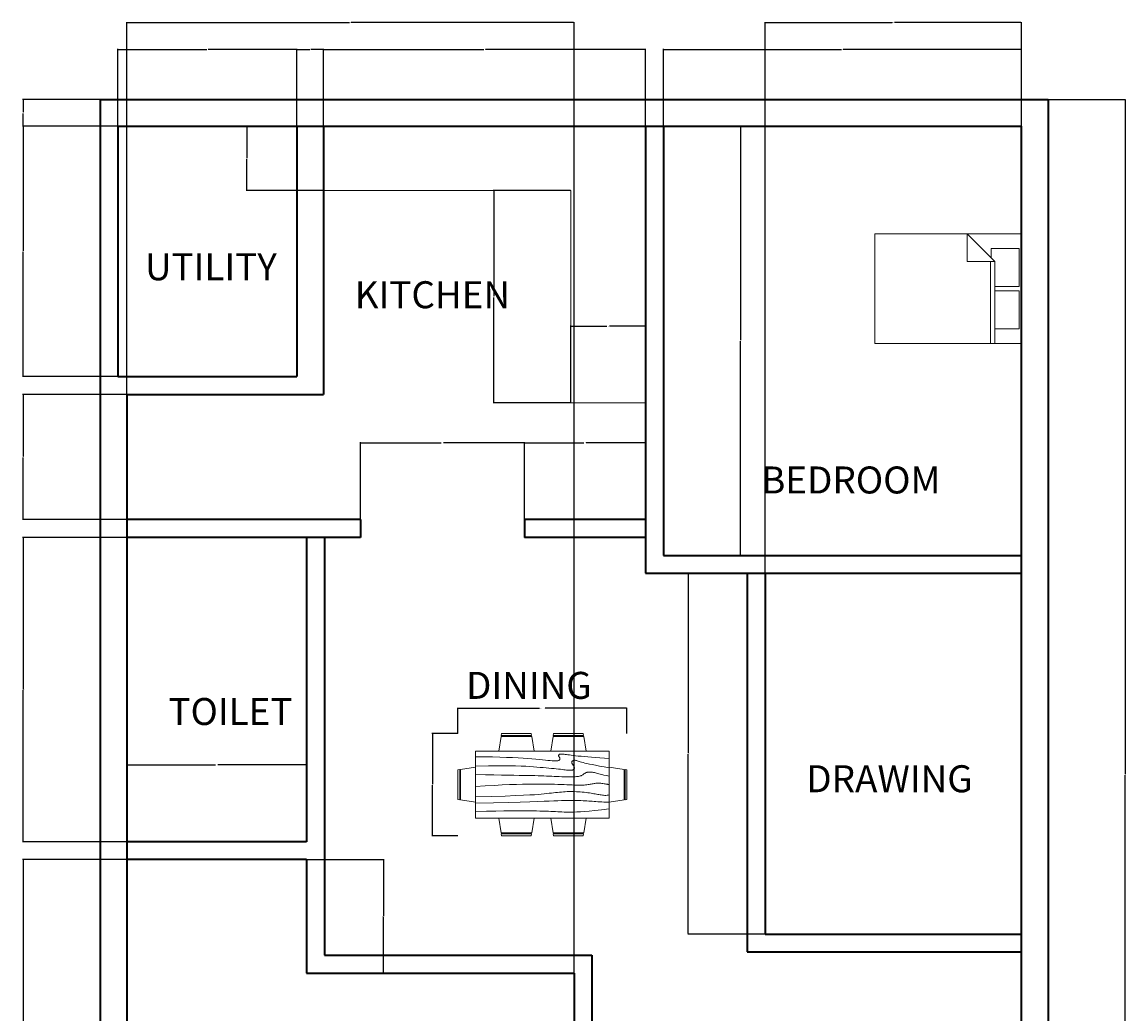
# Model space of a CAD drawing. Units: inches. Extents: x 3024 to 3952, y 1308 to 1863.
# Tile 29 of 29: x 3581 to 3952, y 1481 to 1814. Entities that reach past the tile are written whole.
import ezdxf

# ---------------------------------------------------------------- set-up
doc = ezdxf.new("R2010")
doc.units = ezdxf.units.IN
for name, color, linetype, lineweight in [('A-ANNO-DIMS', 2, 'Continuous', 18), ('A-AREA-IDEN', 7, 'Continuous', 18), ('A-FLOR-CASE', 8, 'Continuous', 18), ('A-FURN', 8, 'Continuous', 18), ('A-WALL', 7, 'Continuous', 35)]:
    doc.layers.add(name, color=color, linetype=linetype, lineweight=lineweight)
doc.styles.get("Standard").update_dxf_attribs({"font": 'arial.ttf'})
doc.dimstyles.get("Standard").update_dxf_attribs({"dimtxt": 0.18, "dimasz": 0.18, "dimexe": 0.18, "dimexo": 0.0625, "dimgap": 0.09, "dimtad": 0, "dimtih": 1, "dimtoh": 1, "dimdec": 4, "dimzin": 0, "dimdsep": 46, "dimtxsty": 'Standard', "dimcen": 0.09, "dimadec": 0, "dimazin": 0, "dimtfac": 1, "dimtdec": 4, "dimtofl": 0, "dimtmove": 0, "dimatfit": 3, "dimfxl": 1, "dimtolj": 1, "dimtzin": 0, "dimarcsym": 0})

# ---------------------------------------------------------------- blocks, each defined once
blk = doc.blocks.new('Bed - Queen')
for p, q in [((0, -80.00003), (0, 0)), ((0, 0), (59.99999, 0)), ((59.99999, 0), (59.99999, -80.00003)), ((7.99999, -1.2), (28.79998, -1.2)), ((7.99999, -14.4), (7.99999, -1.2)), ((28.79998, -1.2), (28.79998, -14.4)), ((31.19999, -1.2), (51.99999, -1.2)), ((31.19999, -14.4), (31.19999, -1.2)), ((51.99999, -1.2), (51.99999, -16.4)), ((0, -14.4), (44.8, -14.4)), ((44.8, -16.8), (0, -16.8)), ((59.99999, -29.6), (44.8, -14.4)), ((44.8, -14.4), (44.8, -29.6)), ((51.99999, -16.4), (46.79936, -16.4)), ((44.8, -29.6), (59.99999, -29.6)), ((59.99999, -80.00003), (0, -80.00003))]:
    blk.add_line(p, q)
blk = doc.blocks.new('Dining Set - 36 x 72 in.')
for p, q in [((-22.2343, 26.00059), (-23.4847, 17.99762)), ((-22.2304, 26), (-5.7608, 26)), ((-22, 27.5), (-22.1562, 26.50042)), ((-5.8416, 26.5), (-22.1534, 26.5)), ((-22, 27.5), (-6, 27.5)), ((-5.8437, 26.49966), (-6, 27.5)), ((-4.5152, 17.99762), (-5.7655, 25.99926)), ((5.7657, 26.00059), (4.5153, 17.99762)), ((5.7696, 26), (22.2392, 26)), ((6, 27.5), (5.8438, 26.50042)), ((22.1584, 26.5), (5.8466, 26.5)), ((6, 27.5), (22, 27.5)), ((22.1563, 26.49966), (22, 27.5)), ((23.4848, 17.99762), (22.2345, 25.99926)), ((36, 18), (-36, 18)), ((-36, 18), (-36, -18)), ((36, -18), (36, 18)), ((-45.5, 8), (-44.5004, 8.15617)), ((-45.5, 8), (-45.5, -8)), ((-44.5, -8.15843), (-44.5, 8.15338)), ((-44.0006, 8.23428), (-35.9976, 9.48474)), ((-44, 8.23041), (-44, -8.23915)), ((44.0006, 8.23428), (35.9976, 9.48474)), ((44, 8.23041), (44, -8.23915)), ((44.5, -8.15843), (44.5, 8.15338)), ((45.5, 8), (44.5005, 8.15617)), ((45.5, 8), (45.5, -8)), ((-44.4997, -8.15631), (-45.5, -8)), ((-35.9976, -9.48476), (-43.9993, -8.2345)), ((35.9976, -9.48476), (43.9993, -8.2345)), ((44.4997, -8.15631), (45.5, -8)), ((-36, -18), (36, -18)), ((-22.2343, -26.0006), (-23.4847, -17.99762)), ((-4.5152, -17.99762), (-5.7655, -25.99928)), ((5.7657, -26.0006), (4.5153, -17.99762)), ((23.4848, -17.99762), (22.2345, -25.99928)), ((-22.2304, -26), (-5.7608, -26)), ((-22, -27.5), (-22.1562, -26.50044)), ((-5.8416, -26.5), (-22.1534, -26.5)), ((-22, -27.5), (-6, -27.5)), ((-5.8437, -26.49967), (-6, -27.5)), ((5.7696, -26), (22.2392, -26)), ((6, -27.5), (5.8438, -26.50044)), ((22.1584, -26.5), (5.8466, -26.5)), ((6, -27.5), (22, -27.5)), ((22.1563, -26.49967), (22, -27.5))]:
    blk.add_line(p, q)
for points in [[(-36, 15), (-31.1772, 14.97754), (-26.8079, 14.91406), (-22.8538, 14.81543), (-19.276, 14.6875), (-16.0362, 14.53613), (-13.0957, 14.36718), (-10.4159, 14.18652), (-7.9583, 14), (-5.6904, 13.81315), (-3.6035, 13.63021), (-1.6954, 13.45508), (0.0365, 13.29166), (1.5945, 13.14388), (2.9811, 13.01562), (4.1988, 12.9108), (5.25, 12.83333), (6.1393, 12.78613), (6.8802, 12.76823), (7.4883, 12.77767), (7.9792, 12.8125), (8.3685, 12.87077), (8.6719, 12.95052), (8.9049, 13.0498), (9.0833, 13.16666), (9.2205, 13.29899), (9.3216, 13.44401), (9.3895, 13.59879), (9.4271, 13.76041), (9.4373, 13.92594), (9.4232, 14.09245), (9.3875, 14.257), (9.3333, 14.41666), (9.2638, 14.56917), (9.1836, 14.71484), (9.0975, 14.85465), (9.0104, 14.98958), (8.9272, 15.1206), (8.8529, 15.2487), (8.7922, 15.37483), (8.75, 15.5), (8.7305, 15.62467), (8.7344, 15.74739), (8.7617, 15.86621), (8.8125, 15.97916), (8.8867, 16.08431), (8.9844, 16.17968), (9.1055, 16.26334), (9.25, 16.33333), (9.4189, 16.38802), (9.6172, 16.42708), (9.8506, 16.45052), (10.125, 16.45833), (10.4463, 16.45052), (10.8203, 16.42708), (11.2529, 16.38802), (11.75, 16.33333), (12.3184, 16.26318), (12.9694, 16.17838), (13.7151, 16.07991), (14.5677, 15.96875), (15.5395, 15.84586), (16.6426, 15.71224), (17.8893, 15.56884), (19.2917, 15.41666), (20.859, 15.25667), (22.5879, 15.08984), (24.4721, 14.91715), (26.5052, 14.73958), (28.6809, 14.5581), (30.9929, 14.3737), (33.4347, 14.18733), (36, 14)], [(-36, 10), (-28.9766, 10.14274), (-23.1725, 10.20442), (-18.4241, 10.19775), (-14.5677, 10.13541), (-11.4399, 10.03011), (-8.877, 9.89453), (-6.7154, 9.74137), (-4.7917, 9.58333), (-2.9698, 9.43082), (-1.2246, 9.28515), (0.4415, 9.14534), (2.026, 9.01041), (3.5266, 8.87939), (4.9408, 8.7513), (6.266, 8.62516), (7.5, 8.5), (8.6411, 8.37549), (9.6914, 8.2539), (10.6538, 8.13818), (11.5312, 8.03125), (12.3267, 7.93603), (13.043, 7.85547), (13.6831, 7.79248), (14.25, 7.75), (14.7471, 7.7303), (15.1797, 7.73307), (15.5537, 7.75732), (15.875, 7.80208), (16.1494, 7.86637), (16.3828, 7.94922), (16.5811, 8.04964), (16.75, 8.16666), (16.8944, 8.29915), (17.0143, 8.44531), (17.1089, 8.60319), (17.1771, 8.77083), (17.218, 8.94629), (17.2305, 9.1276), (17.2137, 9.31282), (17.1667, 9.5), (17.0895, 9.6875), (16.987, 9.875), (16.8649, 10.0625), (16.7292, 10.25), (16.5856, 10.4375), (16.4401, 10.625), (16.2985, 10.8125), (16.1667, 11), (16.05, 11.18733), (15.9518, 11.3737), (15.8752, 11.5581), (15.8229, 11.73958), (15.798, 11.91715), (15.8034, 12.08984), (15.842, 12.25667), (15.9167, 12.41666), (16.0295, 12.56836), (16.1784, 12.70833), (16.3605, 12.83268), (16.5729, 12.9375), (16.8127, 13.01888), (17.0768, 13.07291), (17.3625, 13.0957), (17.6667, 13.08333), (17.9894, 13.03312), (18.3418, 12.94726), (18.7382, 12.82918), (19.1927, 12.68229), (19.7195, 12.51001), (20.3327, 12.31575), (21.0465, 12.10294), (21.875, 11.875), (22.8357, 11.63354), (23.959, 11.37304), (25.2786, 11.08618), (26.8282, 10.76562), (28.6414, 10.40405), (30.752, 9.99414), (33.1936, 9.52856), (36, 9)], [(-36, 5.5), (-30.7157, 5.3348), (-26.069, 5.20963), (-21.9946, 5.11767), (-18.4271, 5.05208), (-15.3009, 5.00602), (-12.5508, 4.97265), (-10.1112, 4.94515), (-7.9167, 4.91666), (-5.909, 4.88167), (-4.0586, 4.83984), (-2.3429, 4.79215), (-0.7396, 4.73958), (0.7739, 4.6831), (2.22, 4.6237), (3.6213, 4.56233), (5, 4.5), (6.373, 4.43782), (7.7344, 4.3776), (9.0723, 4.32129), (10.375, 4.27083), (11.6309, 4.22819), (12.8281, 4.19531), (13.9551, 4.17415), (15, 4.16666), (15.954, 4.17448), (16.819, 4.19791), (17.6001, 4.23698), (18.3021, 4.29166), (18.9299, 4.36198), (19.4883, 4.44791), (19.9823, 4.54948), (20.4167, 4.66666), (20.7969, 4.79899), (21.1302, 4.94401), (21.4245, 5.09879), (21.6875, 5.26041), (21.9271, 5.42594), (22.1511, 5.59245), (22.3672, 5.757), (22.5834, 5.91666), (22.8065, 6.06868), (23.0404, 6.21093), (23.2879, 6.34147), (23.5521, 6.45833), (23.8358, 6.55957), (24.142, 6.64323), (24.4735, 6.70735), (24.8334, 6.75), (25.2235, 6.76969), (25.642, 6.76692), (26.0858, 6.74267), (26.5521, 6.69791), (27.0379, 6.63362), (27.5404, 6.55078), (28.0565, 6.45036), (28.5834, 6.33333), (29.1242, 6.19987), (29.7071, 6.04687), (30.3661, 5.87044), (31.1354, 5.66666), (32.0493, 5.43164), (33.142, 5.16146), (34.4475, 4.85221), (36, 4.5)], [(-36, -1), (-30.7915, -0.6591), (-26.0195, -0.38216), (-21.6519, -0.16284), (-17.6563, 0.00521), (-14.0005, 0.12833), (-10.6523, 0.21289), (-7.5796, 0.26522), (-4.75, 0.29166), (-2.134, 0.29793), (0.2878, 0.28711), (2.5317, 0.26163), (4.6146, 0.22396), (6.5529, 0.17651), (8.3633, 0.12174), (10.0623, 0.06209), (11.6667, 0), (13.1899, -0.06201), (14.6341, -0.1211), (15.9982, -0.17432), (17.2813, -0.21875), (18.4823, -0.25147), (19.6003, -0.26953), (20.6343, -0.27002), (21.5834, -0.25), (22.4481, -0.20768), (23.2357, -0.14584), (23.9549, -0.06836), (24.6146, 0.02083), (25.2235, 0.11784), (25.7904, 0.21875), (26.3241, 0.31966), (26.8334, 0.41666), (27.3265, 0.50618), (27.8099, 0.58593), (28.2894, 0.65397), (28.7709, 0.70833), (29.2601, 0.74707), (29.763, 0.76823), (30.2855, 0.76985), (30.8334, 0.75), (31.4088, 0.70784), (31.9994, 0.64713), (32.589, 0.57275), (33.1615, 0.48958), (33.7008, 0.4025), (34.1908, 0.3164), (34.6153, 0.23616), (34.9584, 0.16666), (35.2099, 0.11165), (35.3848, 0.07031), (35.504, 0.04069), (35.5886, 0.02083), (35.6594, 0.00879), (35.7377, 0.0026), (35.8442, 0.00032), (36, 0)], [(-36, -6.5), (-27.1843, -6.31267), (-20.084, -6.1263), (-14.469, -5.9419), (-10.1094, -5.76042), (-6.7752, -5.58285), (-4.2363, -5.41016), (-2.2629, -5.24333), (-0.625, -5.08334), (0.8708, -4.93099), (2.2715, -4.78646), (3.5872, -4.64974), (4.8281, -4.52084), (6.0046, -4.39974), (7.127, -4.28646), (8.2053, -4.18099), (9.25, -4.08334), (10.2705, -3.99382), (11.2734, -3.91407), (12.2647, -3.84603), (13.25, -3.79167), (14.2354, -3.75293), (15.2266, -3.73177), (16.2295, -3.73015), (17.25, -3.75), (18.2912, -3.79248), (19.3451, -3.85547), (20.4009, -3.93604), (21.4479, -4.03125), (22.4754, -4.13819), (23.4727, -4.25391), (24.4289, -4.37549), (25.3334, -4.5), (26.1785, -4.62492), (26.9694, -4.74935), (27.7145, -4.87281), (28.4219, -4.99479), (29.1, -5.11483), (29.7572, -5.23242), (30.4016, -5.34709), (31.0417, -5.45834), (31.6837, -5.56437), (32.3262, -5.65821), (32.9658, -5.73153), (33.599, -5.77604), (34.2224, -5.78345), (34.8327, -5.74545), (35.4264, -5.65373), (36, -5.5)], [(-36, -10), (-26.4022, -9.81299), (-18.4675, -9.62891), (-11.9839, -9.45069), (-6.7396, -9.28125), (-2.5226, -9.12354), (0.8789, -8.98047), (3.6769, -8.85498), (6.0833, -8.75), (8.2767, -8.66765), (10.3021, -8.60677), (12.1712, -8.56543), (13.8958, -8.54167), (15.4876, -8.53353), (16.9583, -8.53907), (18.3197, -8.55632), (19.5834, -8.58334), (20.7616, -8.61841), (21.8685, -8.66081), (22.9188, -8.71004), (23.9271, -8.76563), (24.9081, -8.82707), (25.8763, -8.89388), (26.8465, -8.96558), (27.8334, -9.04167), (28.8474, -9.12118), (29.8828, -9.20117), (30.93, -9.27824), (31.9792, -9.34896), (33.0205, -9.40991), (34.0443, -9.45768), (35.0407, -9.48885), (36, -9.5)], [(-36, -14.5), (-30.0881, -14.33513), (-25.0332, -14.21224), (-20.7312, -14.12647), (-17.0781, -14.07292), (-13.97, -14.04671), (-11.3027, -14.04297), (-8.9724, -14.05681), (-6.875, -14.08334), (-4.9224, -14.11833), (-3.0905, -14.16016), (-1.3709, -14.20785), (0.2448, -14.26042), (1.7647, -14.3169), (3.1973, -14.3763), (4.5507, -14.43767), (5.8333, -14.5), (7.0554, -14.5621), (8.235, -14.62175), (9.3922, -14.67652), (10.5469, -14.72396), (11.7192, -14.76164), (12.929, -14.78711), (14.1965, -14.79794), (15.5417, -14.79167), (16.9933, -14.76424), (18.6152, -14.70508), (20.4804, -14.60197), (22.6615, -14.44271), (25.2312, -14.21509), (28.2624, -13.9069), (31.8277, -13.50594), (36, -13)]]:
    blk.add_lwpolyline(points)
blk = doc.blocks.new('*D22')
at = {"layer": 'A-ANNO-DIMS', "color": 0, "lineweight": -2, "transparency": 16777216}
for p, q in [((3727.65, 1574.87), (3727.65, 1583.49)), ((3727.83, 1583.31), (3755.04, 1583.31)), ((3784.17, 1583.31), (3756.97, 1583.31)), ((3784.35, 1574.87), (3784.35, 1583.49))]:
    blk.add_line(p, q, dxfattribs=at)
at = {"layer": 'A-ANNO-DIMS', "color": 0, "transparency": 16777216}
for points in [[(3727.83, 1583.34), (3727.83, 1583.28), (3727.65, 1583.31)], [(3784.17, 1583.34), (3784.17, 1583.28), (3784.35, 1583.31)]]:
    blk.add_solid(points, dxfattribs=at)
at = {"layer": 'Defpoints', "color": 0, "transparency": 16777216}
for p in [(3784.35, 1583.31), (3727.65, 1574.81), (3784.35, 1574.81)]:
    blk.add_point(p, dxfattribs=at)
at = {"layer": 'A-ANNO-DIMS', "color": 0, "transparency": 16777216, "insert": (3756, 1583.31), "char_height": 0.18, "attachment_point": 5}
blk.add_mtext('\\A1;DINING SET 57', dxfattribs=at)
blk = doc.blocks.new('*D23')
at = {"layer": 'A-ANNO-DIMS', "color": 0, "lineweight": -2, "transparency": 16777216}
for p, q in [((3727.59, 1574.81), (3718.97, 1574.81)), ((3719.15, 1574.63), (3719.15, 1557.85)), ((3719.15, 1540.72), (3719.15, 1557.49)), ((3727.59, 1540.54), (3718.97, 1540.54))]:
    blk.add_line(p, q, dxfattribs=at)
at = {"layer": 'A-ANNO-DIMS', "color": 0, "transparency": 16777216}
for points in [[(3719.12, 1574.63), (3719.18, 1574.63), (3719.15, 1574.81)], [(3719.12, 1540.72), (3719.18, 1540.72), (3719.15, 1540.54)]]:
    blk.add_solid(points, dxfattribs=at)
at = {"layer": 'Defpoints', "color": 0, "transparency": 16777216}
for p in [(3719.15, 1574.81), (3727.65, 1574.81), (3727.65, 1540.54)]:
    blk.add_point(p, dxfattribs=at)
at = {"layer": 'A-ANNO-DIMS', "color": 0, "transparency": 16777216, "insert": (3719.15, 1557.67), "char_height": 0.18, "attachment_point": 5}
blk.add_mtext('\\A1;34', dxfattribs=at)
blk = doc.blocks.new('*D82')
at = {"layer": 'A-ANNO-DIMS', "color": 0, "lineweight": -2, "transparency": 16777216}
for p, q in [((3925.7, 1787.61), (3951.59, 1787.61)), ((3951.41, 1787.43), (3951.41, 1561.21)), ((3951.41, 1334.62), (3951.41, 1560.84)), ((3925.7, 1334.44), (3951.59, 1334.44))]:
    blk.add_line(p, q, dxfattribs=at)
at = {"layer": 'A-ANNO-DIMS', "color": 0, "transparency": 16777216}
for points in [[(3951.38, 1787.43), (3951.44, 1787.43), (3951.41, 1787.61)], [(3951.38, 1334.62), (3951.44, 1334.62), (3951.41, 1334.44)]]:
    blk.add_solid(points, dxfattribs=at)
at = {"layer": 'Defpoints', "color": 0, "transparency": 16777216}
for p in [(3925.64, 1787.61), (3951.41, 1787.61), (3925.64, 1334.44)]:
    blk.add_point(p, dxfattribs=at)
at = {"layer": 'A-ANNO-DIMS', "color": 0, "transparency": 16777216, "insert": (3951.41, 1561.02), "char_height": 0.18, "attachment_point": 5}
blk.add_mtext('\\A1;453.2', dxfattribs=at)
blk = doc.blocks.new('*D83')
at = {"layer": 'A-ANNO-DIMS', "color": 0, "lineweight": -2, "transparency": 16777216}
for p, q in [((3613.64, 1778.67), (3613.64, 1804.56)), ((3613.82, 1804.38), (3643.42, 1804.38)), ((3673.46, 1804.38), (3643.86, 1804.38)), ((3673.64, 1778.67), (3673.64, 1804.56))]:
    blk.add_line(p, q, dxfattribs=at)
at = {"layer": 'A-ANNO-DIMS', "color": 0, "transparency": 16777216}
for points in [[(3613.82, 1804.41), (3613.82, 1804.35), (3613.64, 1804.38)], [(3673.46, 1804.41), (3673.46, 1804.35), (3673.64, 1804.38)]]:
    blk.add_solid(points, dxfattribs=at)
at = {"layer": 'Defpoints', "color": 0, "transparency": 16777216}
for p in [(3673.64, 1804.38), (3613.64, 1778.61), (3673.64, 1778.61)]:
    blk.add_point(p, dxfattribs=at)
at = {"layer": 'A-ANNO-DIMS', "color": 0, "transparency": 16777216, "insert": (3643.64, 1804.38), "char_height": 0.18, "attachment_point": 5}
blk.add_mtext('\\A1;60', dxfattribs=at)
blk = doc.blocks.new('*D84')
at = {"layer": 'A-ANNO-DIMS', "color": 0, "lineweight": -2, "transparency": 16777216}
for p, q in [((3682.64, 1778.67), (3682.64, 1804.56)), ((3682.82, 1804.38), (3736.36, 1804.38)), ((3790.46, 1804.38), (3736.92, 1804.38)), ((3790.64, 1778.67), (3790.64, 1804.56))]:
    blk.add_line(p, q, dxfattribs=at)
at = {"layer": 'A-ANNO-DIMS', "color": 0, "transparency": 16777216}
for points in [[(3682.82, 1804.41), (3682.82, 1804.35), (3682.64, 1804.38)], [(3790.46, 1804.41), (3790.46, 1804.35), (3790.64, 1804.38)]]:
    blk.add_solid(points, dxfattribs=at)
at = {"layer": 'Defpoints', "color": 0, "transparency": 16777216}
for p in [(3790.64, 1804.38), (3682.64, 1778.61), (3790.64, 1778.61)]:
    blk.add_point(p, dxfattribs=at)
at = {"layer": 'A-ANNO-DIMS', "color": 0, "transparency": 16777216, "insert": (3736.64, 1804.38), "char_height": 0.18, "attachment_point": 5}
blk.add_mtext('\\A1;108', dxfattribs=at)
blk = doc.blocks.new('*D85')
at = {"layer": 'A-ANNO-DIMS', "color": 0, "lineweight": -2, "transparency": 16777216}
for p, q in [((3796.64, 1778.67), (3796.64, 1804.56)), ((3796.82, 1804.38), (3856.36, 1804.38)), ((3916.46, 1804.38), (3856.92, 1804.38)), ((3916.64, 1778.67), (3916.64, 1804.56))]:
    blk.add_line(p, q, dxfattribs=at)
at = {"layer": 'A-ANNO-DIMS', "color": 0, "transparency": 16777216}
for points in [[(3796.82, 1804.41), (3796.82, 1804.35), (3796.64, 1804.38)], [(3916.46, 1804.41), (3916.46, 1804.35), (3916.64, 1804.38)]]:
    blk.add_solid(points, dxfattribs=at)
at = {"layer": 'Defpoints', "color": 0, "transparency": 16777216}
for p in [(3916.64, 1804.38), (3796.64, 1778.61), (3916.64, 1778.61)]:
    blk.add_point(p, dxfattribs=at)
at = {"layer": 'A-ANNO-DIMS', "color": 0, "transparency": 16777216, "insert": (3856.64, 1804.38), "char_height": 0.18, "attachment_point": 5}
blk.add_mtext('\\A1;120', dxfattribs=at)
blk = doc.blocks.new('*D86')
at = {"layer": 'A-ANNO-DIMS', "color": 0, "lineweight": -2, "transparency": 16777216}
for p, q in [((3613.58, 1778.61), (3581.68, 1778.61)), ((3581.86, 1778.43), (3581.86, 1736.79)), ((3581.86, 1694.79), (3581.86, 1736.42)), ((3613.58, 1694.61), (3581.68, 1694.61))]:
    blk.add_line(p, q, dxfattribs=at)
at = {"layer": 'A-ANNO-DIMS', "color": 0, "transparency": 16777216}
for points in [[(3581.83, 1778.43), (3581.89, 1778.43), (3581.86, 1778.61)], [(3581.83, 1694.79), (3581.89, 1694.79), (3581.86, 1694.61)]]:
    blk.add_solid(points, dxfattribs=at)
at = {"layer": 'Defpoints', "color": 0, "transparency": 16777216}
for p in [(3613.64, 1778.61), (3581.86, 1694.61), (3613.64, 1694.61)]:
    blk.add_point(p, dxfattribs=at)
at = {"layer": 'A-ANNO-DIMS', "color": 0, "transparency": 16777216, "insert": (3581.86, 1736.61), "char_height": 0.18, "attachment_point": 5}
blk.add_mtext('\\A1;84', dxfattribs=at)
blk = doc.blocks.new('*D87')
at = {"layer": 'A-ANNO-DIMS', "color": 0, "lineweight": -2, "transparency": 16777216}
for p, q in [((3616.58, 1688.61), (3581.68, 1688.61)), ((3581.86, 1688.43), (3581.86, 1667.79)), ((3581.86, 1646.79), (3581.86, 1667.43)), ((3616.58, 1646.61), (3581.68, 1646.61))]:
    blk.add_line(p, q, dxfattribs=at)
at = {"layer": 'A-ANNO-DIMS', "color": 0, "transparency": 16777216}
for points in [[(3581.83, 1688.43), (3581.89, 1688.43), (3581.86, 1688.61)], [(3581.83, 1646.79), (3581.89, 1646.79), (3581.86, 1646.61)]]:
    blk.add_solid(points, dxfattribs=at)
at = {"layer": 'Defpoints', "color": 0, "transparency": 16777216}
for p in [(3616.64, 1688.61), (3581.86, 1646.61), (3616.64, 1646.61)]:
    blk.add_point(p, dxfattribs=at)
at = {"layer": 'A-ANNO-DIMS', "color": 0, "transparency": 16777216, "insert": (3581.86, 1667.61), "char_height": 0.18, "attachment_point": 5}
blk.add_mtext('\\A1;42', dxfattribs=at)
blk = doc.blocks.new('*D88')
at = {"layer": 'A-ANNO-DIMS', "color": 0, "lineweight": -2, "transparency": 16777216}
for p, q in [((3796.7, 1778.61), (3822.59, 1778.61)), ((3822.41, 1778.43), (3822.41, 1706.79)), ((3822.41, 1634.79), (3822.41, 1706.43)), ((3796.7, 1634.61), (3822.59, 1634.61))]:
    blk.add_line(p, q, dxfattribs=at)
at = {"layer": 'A-ANNO-DIMS', "color": 0, "transparency": 16777216}
for points in [[(3822.38, 1778.43), (3822.44, 1778.43), (3822.41, 1778.61)], [(3822.38, 1634.79), (3822.44, 1634.79), (3822.41, 1634.61)]]:
    blk.add_solid(points, dxfattribs=at)
at = {"layer": 'Defpoints', "color": 0, "transparency": 16777216}
for p in [(3796.64, 1778.61), (3796.64, 1634.61), (3822.41, 1634.61)]:
    blk.add_point(p, dxfattribs=at)
at = {"layer": 'A-ANNO-DIMS', "color": 0, "transparency": 16777216, "insert": (3822.41, 1706.61), "char_height": 0.18, "attachment_point": 5}
blk.add_mtext('\\A1;144', dxfattribs=at)
blk = doc.blocks.new('*D89')
at = {"layer": 'A-ANNO-DIMS', "color": 0, "lineweight": -2, "transparency": 16777216}
for p, q in [((3830.66, 1628.61), (3804.77, 1628.61)), ((3804.95, 1628.43), (3804.95, 1568.25)), ((3804.95, 1507.7), (3804.95, 1567.88)), ((3830.66, 1507.52), (3804.77, 1507.52))]:
    blk.add_line(p, q, dxfattribs=at)
at = {"layer": 'A-ANNO-DIMS', "color": 0, "transparency": 16777216}
for points in [[(3804.92, 1628.43), (3804.98, 1628.43), (3804.95, 1628.61)], [(3804.92, 1507.7), (3804.98, 1507.7), (3804.95, 1507.52)]]:
    blk.add_solid(points, dxfattribs=at)
at = {"layer": 'Defpoints', "color": 0, "transparency": 16777216}
for p in [(3804.95, 1628.61), (3830.72, 1628.61), (3830.72, 1507.52)]:
    blk.add_point(p, dxfattribs=at)
at = {"layer": 'A-ANNO-DIMS', "color": 0, "transparency": 16777216, "insert": (3804.95, 1568.06), "char_height": 0.18, "attachment_point": 5}
blk.add_mtext('\\A1;121.08', dxfattribs=at)
blk = doc.blocks.new('*D90')
at = {"layer": 'A-ANNO-DIMS', "color": 0, "lineweight": -2, "transparency": 16777216}
for p, q in [((3830.72, 1507.58), (3830.72, 1813.56)), ((3830.9, 1813.38), (3873.29, 1813.38)), ((3916.46, 1813.38), (3874.07, 1813.38)), ((3916.64, 1507.58), (3916.64, 1813.56))]:
    blk.add_line(p, q, dxfattribs=at)
at = {"layer": 'A-ANNO-DIMS', "color": 0, "transparency": 16777216}
for points in [[(3830.9, 1813.41), (3830.9, 1813.35), (3830.72, 1813.38)], [(3916.46, 1813.41), (3916.46, 1813.35), (3916.64, 1813.38)]]:
    blk.add_solid(points, dxfattribs=at)
at = {"layer": 'Defpoints', "color": 0, "transparency": 16777216}
for p in [(3916.64, 1813.38), (3830.72, 1507.52), (3916.64, 1507.52)]:
    blk.add_point(p, dxfattribs=at)
at = {"layer": 'A-ANNO-DIMS', "color": 0, "transparency": 16777216, "insert": (3873.68, 1813.38), "char_height": 0.18, "attachment_point": 5}
blk.add_mtext('\\A1;85.92', dxfattribs=at)
blk = doc.blocks.new('*D91')
at = {"layer": 'A-ANNO-DIMS', "color": 0, "lineweight": -2, "transparency": 16777216}
for p, q in [((3616.64, 1538.58), (3616.64, 1564.48)), ((3616.82, 1564.3), (3646.39, 1564.3)), ((3676.74, 1564.3), (3647.17, 1564.3)), ((3676.92, 1538.58), (3676.92, 1564.48))]:
    blk.add_line(p, q, dxfattribs=at)
at = {"layer": 'A-ANNO-DIMS', "color": 0, "transparency": 16777216}
for points in [[(3616.82, 1564.33), (3616.82, 1564.27), (3616.64, 1564.3)], [(3676.74, 1564.33), (3676.74, 1564.27), (3676.92, 1564.3)]]:
    blk.add_solid(points, dxfattribs=at)
at = {"layer": 'Defpoints', "color": 0, "transparency": 16777216}
for p in [(3676.92, 1564.3), (3616.64, 1538.52), (3676.92, 1538.52)]:
    blk.add_point(p, dxfattribs=at)
at = {"layer": 'A-ANNO-DIMS', "color": 0, "transparency": 16777216, "insert": (3646.78, 1564.3), "char_height": 0.18, "attachment_point": 5}
blk.add_mtext('\\A1;60.28', dxfattribs=at)
blk = doc.blocks.new('*D92')
at = {"layer": 'A-ANNO-DIMS', "color": 0, "lineweight": -2, "transparency": 16777216}
for p, q in [((3616.58, 1640.61), (3581.68, 1640.61)), ((3581.86, 1640.43), (3581.86, 1589.75)), ((3581.86, 1538.7), (3581.86, 1589.38)), ((3616.58, 1538.52), (3581.68, 1538.52))]:
    blk.add_line(p, q, dxfattribs=at)
at = {"layer": 'A-ANNO-DIMS', "color": 0, "transparency": 16777216}
for points in [[(3581.83, 1640.43), (3581.89, 1640.43), (3581.86, 1640.61)], [(3581.83, 1538.7), (3581.89, 1538.7), (3581.86, 1538.52)]]:
    blk.add_solid(points, dxfattribs=at)
at = {"layer": 'Defpoints', "color": 0, "transparency": 16777216}
for p in [(3616.64, 1640.61), (3581.86, 1538.52), (3616.64, 1538.52)]:
    blk.add_point(p, dxfattribs=at)
at = {"layer": 'A-ANNO-DIMS', "color": 0, "transparency": 16777216, "insert": (3581.86, 1589.56), "char_height": 0.18, "attachment_point": 5}
blk.add_mtext('\\A1;102.08', dxfattribs=at)
blk = doc.blocks.new('*D93')
at = {"layer": 'A-ANNO-DIMS', "color": 0, "lineweight": -2, "transparency": 16777216}
for p, q in [((3616.64, 1343.5), (3616.64, 1813.56)), ((3616.82, 1813.38), (3691.36, 1813.38)), ((3766.46, 1813.38), (3691.92, 1813.38)), ((3766.64, 1343.5), (3766.64, 1813.56))]:
    blk.add_line(p, q, dxfattribs=at)
at = {"layer": 'A-ANNO-DIMS', "color": 0, "transparency": 16777216}
for points in [[(3616.82, 1813.41), (3616.82, 1813.35), (3616.64, 1813.38)], [(3766.46, 1813.41), (3766.46, 1813.35), (3766.64, 1813.38)]]:
    blk.add_solid(points, dxfattribs=at)
at = {"layer": 'Defpoints', "color": 0, "transparency": 16777216}
for p in [(3766.64, 1813.38), (3616.64, 1343.44), (3766.64, 1343.44)]:
    blk.add_point(p, dxfattribs=at)
at = {"layer": 'A-ANNO-DIMS', "color": 0, "transparency": 16777216, "insert": (3691.64, 1813.38), "char_height": 0.18, "attachment_point": 5}
blk.add_mtext('\\A1;150', dxfattribs=at)
blk = doc.blocks.new('*D94')
at = {"layer": 'A-ANNO-DIMS', "color": 0, "lineweight": -2, "transparency": 16777216}
for p, q in [((3676.98, 1532.52), (3702.88, 1532.52)), ((3702.7, 1532.34), (3702.7, 1513.67)), ((3702.7, 1494.63), (3702.7, 1513.31)), ((3676.98, 1494.45), (3702.88, 1494.45))]:
    blk.add_line(p, q, dxfattribs=at)
at = {"layer": 'A-ANNO-DIMS', "color": 0, "transparency": 16777216}
for points in [[(3702.67, 1532.34), (3702.73, 1532.34), (3702.7, 1532.52)], [(3702.67, 1494.63), (3702.73, 1494.63), (3702.7, 1494.45)]]:
    blk.add_solid(points, dxfattribs=at)
at = {"layer": 'Defpoints', "color": 0, "transparency": 16777216}
for p in [(3676.92, 1532.52), (3676.92, 1494.45), (3702.7, 1494.45)]:
    blk.add_point(p, dxfattribs=at)
at = {"layer": 'A-ANNO-DIMS', "color": 0, "transparency": 16777216, "insert": (3702.7, 1513.49), "char_height": 0.18, "attachment_point": 5}
blk.add_mtext('\\A1;38.07', dxfattribs=at)
blk = doc.blocks.new('*D95')
at = {"layer": 'A-ANNO-DIMS', "color": 0, "lineweight": -2, "transparency": 16777216}
for p, q in [((3694.98, 1646.67), (3694.98, 1672.56)), ((3695.16, 1672.38), (3722.1, 1672.38)), ((3749.82, 1672.38), (3722.88, 1672.38)), ((3750, 1646.67), (3750, 1672.56))]:
    blk.add_line(p, q, dxfattribs=at)
at = {"layer": 'A-ANNO-DIMS', "color": 0, "transparency": 16777216}
for points in [[(3695.16, 1672.41), (3695.16, 1672.35), (3694.98, 1672.38)], [(3749.82, 1672.41), (3749.82, 1672.35), (3750, 1672.38)]]:
    blk.add_solid(points, dxfattribs=at)
at = {"layer": 'Defpoints', "color": 0, "transparency": 16777216}
for p in [(3750, 1672.38), (3694.98, 1646.61), (3750, 1646.61)]:
    blk.add_point(p, dxfattribs=at)
at = {"layer": 'A-ANNO-DIMS', "color": 0, "transparency": 16777216, "insert": (3722.49, 1672.38), "char_height": 0.18, "attachment_point": 5}
blk.add_mtext('\\A1;55.03', dxfattribs=at)
blk = doc.blocks.new('*D96')
at = {"layer": 'A-ANNO-DIMS', "color": 0, "lineweight": -2, "transparency": 16777216}
for p, q in [((3750, 1646.67), (3750, 1672.56)), ((3750.18, 1672.38), (3769.92, 1672.38)), ((3790.46, 1672.38), (3770.72, 1672.38)), ((3790.64, 1646.67), (3790.64, 1672.56))]:
    blk.add_line(p, q, dxfattribs=at)
at = {"layer": 'A-ANNO-DIMS', "color": 0, "transparency": 16777216}
for points in [[(3750.18, 1672.41), (3750.18, 1672.35), (3750, 1672.38)], [(3790.46, 1672.41), (3790.46, 1672.35), (3790.64, 1672.38)]]:
    blk.add_solid(points, dxfattribs=at)
at = {"layer": 'Defpoints', "color": 0, "transparency": 16777216}
for p in [(3790.64, 1672.38), (3750, 1646.61), (3790.64, 1646.61)]:
    blk.add_point(p, dxfattribs=at)
at = {"layer": 'A-ANNO-DIMS', "color": 0, "transparency": 16777216, "insert": (3770.32, 1672.38), "char_height": 0.18, "attachment_point": 5}
blk.add_mtext('\\A1;40.63', dxfattribs=at)
blk = doc.blocks.new('*D97')
at = {"layer": 'A-ANNO-DIMS', "color": 0, "lineweight": -2, "transparency": 16777216}
for p, q in [((3616.58, 1532.52), (3581.68, 1532.52)), ((3581.86, 1532.34), (3581.86, 1438.16)), ((3581.86, 1343.62), (3581.86, 1437.8)), ((3616.58, 1343.44), (3581.68, 1343.44))]:
    blk.add_line(p, q, dxfattribs=at)
at = {"layer": 'A-ANNO-DIMS', "color": 0, "transparency": 16777216}
for points in [[(3581.83, 1532.34), (3581.89, 1532.34), (3581.86, 1532.52)], [(3581.83, 1343.62), (3581.89, 1343.62), (3581.86, 1343.44)]]:
    blk.add_solid(points, dxfattribs=at)
at = {"layer": 'Defpoints', "color": 0, "transparency": 16777216}
for p in [(3581.86, 1532.52), (3616.64, 1532.52), (3616.64, 1343.44)]:
    blk.add_point(p, dxfattribs=at)
at = {"layer": 'A-ANNO-DIMS', "color": 0, "transparency": 16777216, "insert": (3581.86, 1437.98), "char_height": 0.18, "attachment_point": 5}
blk.add_mtext('\\A1;189.1', dxfattribs=at)
blk = doc.blocks.new('*D98')
at = {"layer": 'A-ANNO-DIMS', "color": 0, "lineweight": -2, "transparency": 16777216}
for p, q in [((3765.5, 1685.8), (3765.5, 1711.69)), ((3765.68, 1711.51), (3777.67, 1711.51)), ((3790.46, 1711.51), (3778.46, 1711.51)), ((3790.64, 1685.8), (3790.64, 1711.69))]:
    blk.add_line(p, q, dxfattribs=at)
at = {"layer": 'A-ANNO-DIMS', "color": 0, "transparency": 16777216}
for points in [[(3765.68, 1711.54), (3765.68, 1711.48), (3765.5, 1711.51)], [(3790.46, 1711.54), (3790.46, 1711.48), (3790.64, 1711.51)]]:
    blk.add_solid(points, dxfattribs=at)
at = {"layer": 'Defpoints', "color": 0, "transparency": 16777216}
for p in [(3790.64, 1711.51), (3765.5, 1685.74), (3790.64, 1685.74)]:
    blk.add_point(p, dxfattribs=at)
at = {"layer": 'A-ANNO-DIMS', "color": 0, "transparency": 16777216, "insert": (3778.07, 1711.51), "char_height": 0.18, "attachment_point": 5}
blk.add_mtext('\\A1;25.14', dxfattribs=at)
blk = doc.blocks.new('*D99')
at = {"layer": 'A-ANNO-DIMS', "color": 0, "lineweight": -2, "transparency": 16777216}
for p, q in [((3765.43, 1757.01), (3739.54, 1757.01)), ((3739.72, 1756.83), (3739.72, 1721.55)), ((3739.72, 1685.92), (3739.72, 1721.19)), ((3765.43, 1685.74), (3739.54, 1685.74))]:
    blk.add_line(p, q, dxfattribs=at)
at = {"layer": 'A-ANNO-DIMS', "color": 0, "transparency": 16777216}
for points in [[(3739.69, 1756.83), (3739.75, 1756.83), (3739.72, 1757.01)], [(3739.69, 1685.92), (3739.75, 1685.92), (3739.72, 1685.74)]]:
    blk.add_solid(points, dxfattribs=at)
at = {"layer": 'Defpoints', "color": 0, "transparency": 16777216}
for p in [(3739.72, 1757.01), (3765.5, 1757.01), (3765.5, 1685.74)]:
    blk.add_point(p, dxfattribs=at)
at = {"layer": 'A-ANNO-DIMS', "color": 0, "transparency": 16777216, "insert": (3739.72, 1721.37), "char_height": 0.18, "attachment_point": 5}
blk.add_mtext('\\A1;71.27', dxfattribs=at)
blk = doc.blocks.new('*D100')
at = {"layer": 'A-ANNO-DIMS', "color": 0, "lineweight": -2, "transparency": 16777216}
for p, q in [((3682.58, 1778.61), (3656.68, 1778.61)), ((3656.86, 1778.43), (3656.86, 1767.99)), ((3656.86, 1757.19), (3656.86, 1767.63)), ((3682.58, 1757.01), (3656.68, 1757.01))]:
    blk.add_line(p, q, dxfattribs=at)
at = {"layer": 'A-ANNO-DIMS', "color": 0, "transparency": 16777216}
for points in [[(3656.83, 1778.43), (3656.89, 1778.43), (3656.86, 1778.61)], [(3656.83, 1757.19), (3656.89, 1757.19), (3656.86, 1757.01)]]:
    blk.add_solid(points, dxfattribs=at)
at = {"layer": 'Defpoints', "color": 0, "transparency": 16777216}
for p in [(3656.86, 1778.61), (3682.64, 1778.61), (3682.64, 1757.01)]:
    blk.add_point(p, dxfattribs=at)
at = {"layer": 'A-ANNO-DIMS', "color": 0, "transparency": 16777216, "insert": (3656.86, 1767.81), "char_height": 0.18, "attachment_point": 5}
blk.add_mtext('\\A1;21.6', dxfattribs=at)
blk = doc.blocks.new('*D101')
at = {"layer": 'A-ANNO-DIMS', "color": 0, "lineweight": -2, "transparency": 16777216}
for p, q in [((3673.64, 1778.67), (3673.64, 1804.56)), ((3673.82, 1804.38), (3677.99, 1804.38)), ((3682.46, 1804.38), (3678.29, 1804.38)), ((3682.64, 1778.67), (3682.64, 1804.56))]:
    blk.add_line(p, q, dxfattribs=at)
at = {"layer": 'A-ANNO-DIMS', "color": 0, "transparency": 16777216}
for points in [[(3673.82, 1804.41), (3673.82, 1804.35), (3673.64, 1804.38)], [(3682.46, 1804.41), (3682.46, 1804.35), (3682.64, 1804.38)]]:
    blk.add_solid(points, dxfattribs=at)
at = {"layer": 'Defpoints', "color": 0, "transparency": 16777216}
for p in [(3682.64, 1804.38), (3673.64, 1778.61), (3682.64, 1778.61)]:
    blk.add_point(p, dxfattribs=at)
at = {"layer": 'A-ANNO-DIMS', "color": 0, "transparency": 16777216, "insert": (3678.14, 1804.38), "char_height": 0.18, "attachment_point": 5}
blk.add_mtext('\\A1;9', dxfattribs=at)
blk = doc.blocks.new('*D103')
at = {"layer": 'A-ANNO-DIMS', "color": 0, "lineweight": -2, "transparency": 16777216}
for p, q in [((3607.58, 1787.61), (3581.68, 1787.61)), ((3581.86, 1787.43), (3581.86, 1783.29)), ((3581.86, 1778.79), (3581.86, 1782.92)), ((3613.58, 1778.61), (3581.68, 1778.61))]:
    blk.add_line(p, q, dxfattribs=at)
at = {"layer": 'A-ANNO-DIMS', "color": 0, "transparency": 16777216}
for points in [[(3581.83, 1787.43), (3581.89, 1787.43), (3581.86, 1787.61)], [(3581.83, 1778.79), (3581.89, 1778.79), (3581.86, 1778.61)]]:
    blk.add_solid(points, dxfattribs=at)
at = {"layer": 'Defpoints', "color": 0, "transparency": 16777216}
for p in [(3607.64, 1787.61), (3581.86, 1778.61), (3613.64, 1778.61)]:
    blk.add_point(p, dxfattribs=at)
at = {"layer": 'A-ANNO-DIMS', "color": 0, "transparency": 16777216, "insert": (3581.86, 1783.11), "char_height": 0.18, "attachment_point": 5}
blk.add_mtext('\\A1;9', dxfattribs=at)

msp = doc.modelspace()

# ---------------------------------------------------------------- linework, layer by layer
at = {"layer": 'A-FLOR-CASE'}
for p, q in [((3682.6376, 1757.0081), (3765.496, 1757.0081)), ((3765.496, 1757.0081), (3765.496, 1685.7374)), ((3765.496, 1685.7374), (3790.6376, 1685.7374))]:
    msp.add_line(p, q, dxfattribs=at)
at = {"layer": 'A-WALL'}
for p, q in [((3607.6376, 1787.6064), (3607.6376, 1334.4405)), ((3607.6376, 1787.6064), (3925.6376, 1787.6064)), ((3925.6376, 1787.6064), (3925.6376, 1334.4405)), ((3613.6376, 1778.6064), (3613.6376, 1694.6064)), ((3613.6376, 1778.6064), (3916.6376, 1778.6064)), ((3673.6376, 1778.6064), (3673.6376, 1694.6064)), ((3682.6376, 1778.6064), (3682.6376, 1688.6064)), ((3790.6376, 1778.6064), (3790.6376, 1628.6064)), ((3796.6376, 1778.6064), (3796.6376, 1634.6064)), ((3916.6376, 1778.6064), (3916.6376, 1484.6064)), ((3613.6376, 1694.6064), (3673.6376, 1694.6064)), ((3616.6376, 1688.6064), (3682.6376, 1688.6064)), ((3616.6376, 1688.6064), (3616.6376, 1343.4405)), ((3694.9779, 1646.6064), (3616.6376, 1646.6064)), ((3694.9779, 1646.6064), (3694.9779, 1640.6064)), ((3790.6376, 1646.6064), (3750.0046, 1646.6064)), ((3750.0046, 1646.6064), (3750.0046, 1640.6064)), ((3694.9779, 1640.6064), (3616.6376, 1640.6064)), ((3676.9212, 1640.6064), (3676.9212, 1538.5223)), ((3682.9212, 1640.6064), (3682.9212, 1532.5223)), ((3790.6376, 1640.6064), (3750.0046, 1640.6064)), ((3796.6376, 1634.6064), (3916.6376, 1634.6064)), ((3790.6376, 1628.6064), (3916.6376, 1628.6064)), ((3824.7207, 1628.6064), (3824.7207, 1501.5221)), ((3830.7207, 1628.6064), (3830.7207, 1507.5221)), ((3676.9212, 1538.5223), (3616.6376, 1538.5223)), ((3676.9212, 1532.5223), (3616.6376, 1532.5223)), ((3676.9212, 1532.5223), (3676.9212, 1494.4537)), ((3682.9212, 1532.5223), (3682.9212, 1500.4537)), ((3830.7207, 1507.5221), (3916.6376, 1507.5221)), ((3682.9212, 1500.4537), (3772.6376, 1500.4537)), ((3772.6376, 1500.4537), (3772.6376, 1343.4405)), ((3824.7207, 1501.5221), (3916.6376, 1501.5221)), ((3916.6376, 1501.5221), (3916.6376, 1343.4405)), ((3676.9212, 1494.4537), (3766.6376, 1494.4537)), ((3766.6376, 1494.4537), (3766.6376, 1343.4405))]:
    msp.add_line(p, q, dxfattribs=at)

# ---------------------------------------------------------------- block references
at = {"layer": 'A-FURN', "xscale": -0.613989453470478, "yscale": 0.613989453470478, "zscale": 0.613989453470478, "rotation": 270.0000000000007}
msp.add_blockref('Bed - Queen', (3916.6376, 1705.6618), dxfattribs=at)
at = {"layer": 'A-FURN', "xscale": 0.6230770906043281, "yscale": 0.6230770906043281, "zscale": 0.6230770906043281}
msp.add_blockref('Dining Set - 36 x 72 in.', (3756.0043, 1557.673), dxfattribs=at)

# ---------------------------------------------------------------- texts
at = {"layer": 'A-AREA-IDEN'}
for s, p in [('UTILITY', (3622.7089, 1726.9194)), ('KITCHEN', (3693.0636, 1717.5318)), ('BEDROOM', (3829.3816, 1655.3692)), ('DINING', (3730.3991, 1586.4463)), ('TOILET', (3630.592, 1577.6781)), ('DRAWING', (3844.5213, 1555.1115))]:
    msp.add_text(s, height=9.05874, dxfattribs=at).set_placement(p)

# ---------------------------------------------------------------- dimensions: what is measured, and where the dimension line sits
at = {"layer": 'A-ANNO-DIMS'}
for base, p1, p2, override, picture, middle in [((3766.6376, 1813.3814), (3616.6376, 1343.4405), (3766.6376, 1343.4405), {"dimdec": 0, "dimlfac": 1, "dimrnd": 0, "dimzin": 0, "dimdsep": 46, "dimlunit": 2}, '*D93', (3691.6376, 1813.3814)), ((3916.6376, 1813.3814), (3830.7207, 1507.5221), (3916.6376, 1507.5221), {"dimdec": 2, "dimlfac": 1, "dimrnd": 0, "dimzin": 0, "dimdsep": 46, "dimlunit": 2}, '*D90', (3873.6791, 1813.3814)), ((3673.6376, 1804.3814), (3613.6376, 1778.6064), (3673.6376, 1778.6064), {"dimdec": 0, "dimlfac": 1, "dimrnd": 0, "dimzin": 0, "dimdsep": 46, "dimlunit": 2}, '*D83', (3643.6376, 1804.3814)), ((3682.6376, 1804.3814), (3673.6376, 1778.6064), (3682.6376, 1778.6064), {"dimdec": 0, "dimlfac": 1, "dimrnd": 0, "dimzin": 0, "dimdsep": 46, "dimlunit": 2}, '*D101', (3678.1376, 1804.3814)), ((3790.6376, 1804.3814), (3682.6376, 1778.6064), (3790.6376, 1778.6064), {"dimdec": 0, "dimlfac": 1, "dimrnd": 0, "dimzin": 0, "dimdsep": 46, "dimlunit": 2}, '*D84', (3736.6376, 1804.3814)), ((3916.6376, 1804.3814), (3796.6376, 1778.6064), (3916.6376, 1778.6064), {"dimdec": 0, "dimlfac": 1, "dimrnd": 0, "dimzin": 0, "dimdsep": 46, "dimlunit": 2}, '*D85', (3856.6376, 1804.3814)), ((3790.6376, 1711.5124), (3765.496, 1685.7374), (3790.6376, 1685.7374), {"dimdec": 2, "dimlfac": 1, "dimrnd": 0, "dimzin": 0, "dimdsep": 46, "dimlunit": 2}, '*D98', (3778.0668, 1711.5124)), ((3790.6376, 1672.3814), (3750.0046, 1646.6064), (3790.6376, 1646.6064), {"dimdec": 2, "dimlfac": 1, "dimrnd": 0, "dimzin": 0, "dimdsep": 46, "dimlunit": 2}, '*D96', (3770.3211, 1672.3814)), ((3676.9212, 1564.2973), (3616.6376, 1538.5223), (3676.9212, 1538.5223), {"dimdec": 2, "dimlfac": 1, "dimrnd": 0, "dimzin": 0, "dimdsep": 46, "dimlunit": 2}, '*D91', (3646.7794, 1564.2973))]:
    dim = msp.add_linear_dim(base=base, p1=p1, p2=p2, dimstyle='Standard', override=override, dxfattribs=at)
    dim.commit()
    dim.dimension.update_dxf_attribs({"geometry": picture, "text_midpoint": middle})
for base, p1, p2, angle, override, picture, middle in [((3581.8626, 1778.6064), (3607.6376, 1787.6064), (3613.6376, 1778.6064), 90, {"dimdec": 0, "dimlfac": 1, "dimrnd": 0, "dimzin": 0, "dimdsep": 46, "dimlunit": 2}, '*D103', (3581.8626, 1783.1064)), ((3951.4126, 1787.6064), (3925.6376, 1334.4405), (3925.6376, 1787.6064), 90, {"dimdec": 1, "dimlfac": 1, "dimrnd": 0, "dimzin": 0, "dimdsep": 46, "dimlunit": 2}, '*D82', (3951.4126, 1561.0234)), ((3581.8626, 1694.6064), (3613.6376, 1778.6064), (3613.6376, 1694.6064), 90, {"dimdec": 0, "dimlfac": 1, "dimrnd": 0, "dimzin": 0, "dimdsep": 46, "dimlunit": 2}, '*D86', (3581.8626, 1736.6064)), ((3656.8626, 1778.6064), (3682.6376, 1757.0081), (3682.6376, 1778.6064), 90, {"dimdec": 1, "dimlfac": 1, "dimrnd": 0, "dimzin": 0, "dimdsep": 46, "dimlunit": 2}, '*D100', (3656.8626, 1767.8073)), ((3822.4126, 1634.6064), (3796.6376, 1778.6064), (3796.6376, 1634.6064), 270, {"dimdec": 0, "dimlfac": 1, "dimrnd": 0, "dimzin": 0, "dimdsep": 46, "dimlunit": 2}, '*D88', (3822.4126, 1706.6064)), ((3739.721, 1757.0081), (3765.496, 1685.7374), (3765.496, 1757.0081), 90, {"dimdec": 2, "dimlfac": 1, "dimrnd": 0, "dimzin": 0, "dimdsep": 46, "dimlunit": 2}, '*D99', (3739.721, 1721.3728)), ((3581.8626, 1646.6064), (3616.6376, 1688.6064), (3616.6376, 1646.6064), 90, {"dimdec": 0, "dimlfac": 1, "dimrnd": 0, "dimzin": 0, "dimdsep": 46, "dimlunit": 2}, '*D87', (3581.8626, 1667.6064)), ((3750.0046, 1672.3814), (3694.9779, 1646.6064), (3750.0046, 1646.6064), 0, {"dimdec": 2, "dimlfac": 1, "dimrnd": 0, "dimzin": 0, "dimdsep": 46, "dimlunit": 2}, '*D95', (3722.4913, 1672.3814)), ((3581.8626, 1538.5223), (3616.6376, 1640.6064), (3616.6376, 1538.5223), 90, {"dimdec": 2, "dimlfac": 1, "dimrnd": 0, "dimzin": 0, "dimdsep": 46, "dimlunit": 2}, '*D92', (3581.8626, 1589.5644)), ((3804.9457, 1628.6064), (3830.7207, 1507.5221), (3830.7207, 1628.6064), 90, {"dimdec": 2, "dimlfac": 1, "dimrnd": 0, "dimzin": 0, "dimdsep": 46, "dimlunit": 2}, '*D89', (3804.9457, 1568.0643)), ((3719.1493, 1574.8076), (3727.6543, 1540.5384), (3727.6543, 1574.8076), 90, {"dimdec": 0, "dimlfac": 1, "dimrnd": 0, "dimzin": 0, "dimdsep": 46, "dimlunit": 2}, '*D23', (3719.1493, 1557.673)), ((3581.8626, 1532.5223), (3616.6376, 1343.4405), (3616.6376, 1532.5223), 90, {"dimdec": 1, "dimlfac": 1, "dimrnd": 0, "dimzin": 0, "dimdsep": 46, "dimlunit": 2}, '*D97', (3581.8626, 1437.9814)), ((3702.6962, 1494.4537), (3676.9212, 1532.5223), (3676.9212, 1494.4537), 270, {"dimdec": 2, "dimlfac": 1, "dimrnd": 0, "dimzin": 0, "dimdsep": 46, "dimlunit": 2}, '*D94', (3702.6962, 1513.488))]:
    dim = msp.add_linear_dim(base=base, p1=p1, p2=p2, angle=angle, dimstyle='Standard', override=override, dxfattribs=at)
    dim.commit()
    dim.dimension.update_dxf_attribs({"geometry": picture, "text_midpoint": middle})
dim = msp.add_linear_dim(base=(3784.3543, 1583.3126), p1=(3727.6543, 1574.8076), p2=(3784.3543, 1574.8076), text='DINING SET <>', dimstyle='Standard', override={"dimdec": 0, "dimlfac": 1, "dimrnd": 0, "dimzin": 0, "dimdsep": 46, "dimlunit": 2}, dxfattribs=at)
dim.commit()
dim.dimension.update_dxf_attribs({"geometry": '*D22', "text_midpoint": (3756.0043, 1583.3126)})

doc.saveas('drawing.dxf')
